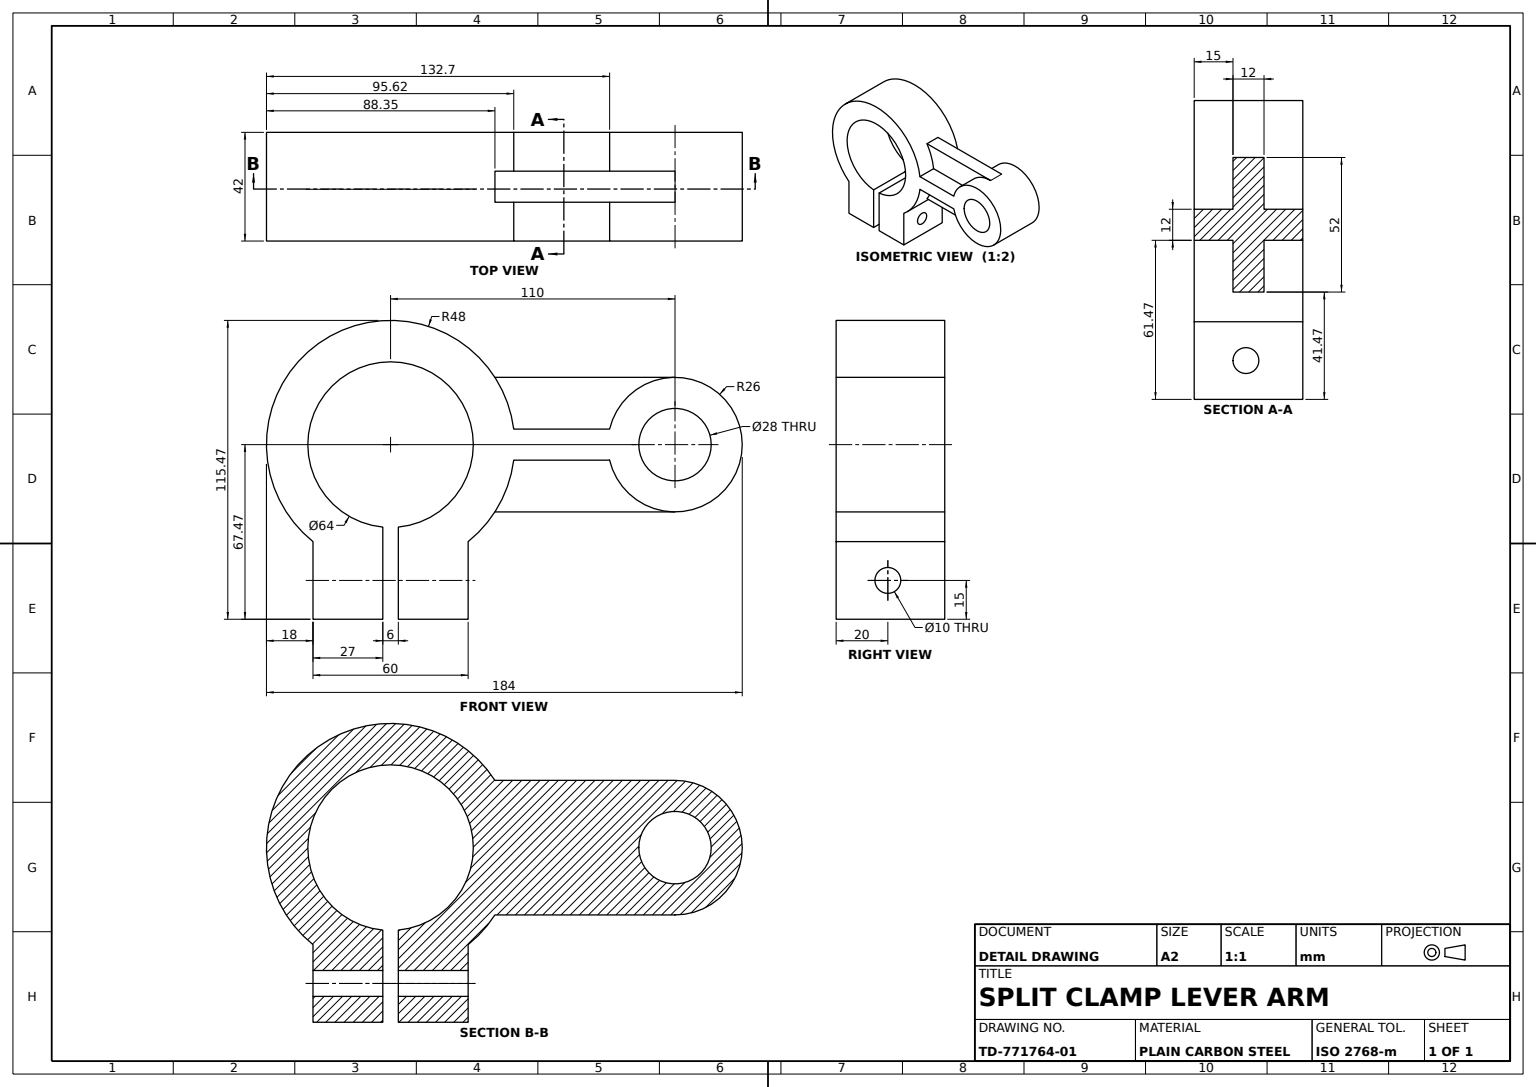
from build123d import *

# Parameters (mm, degrees)
CLAMP_BODY_DEPTH          = 40
CLAMP_BODY_DEPTH_BACK     = 2
CLAMP_SCREW_HOLE_SKETCH_R = 5
CLAMP_SCREW_HOLE_10_DEPTH = 111.617355236
PIVOT_ARM_SKETCH_R        = 14
PIVOT_ARM_AND_BOSS_DEPTH  = 42
ARM_RIB_REACH             = 171.802
ARM_RIB_SKETCH_WALLS_W    = 433.168174749
ARM_RIB_SKETCH_WALLS_H    = 12
CLAMP_RIB_REACH           = 161.912
CLAMP_RIB_SKETCH_WALLS_W  = 402.175841481
CLAMP_RIB_SKETCH_WALLS_H  = 12
BORE_START                = -60
BORE_SKETCH_R             = 32
BORE_64_DEPTH             = 60


with BuildPart() as part:
    # Clamp Body Sketch → Clamp Body (new, two sides: drawn at the far end of the back side and taken through both)
    with BuildSketch(Plane.XY.offset(-CLAMP_BODY_DEPTH_BACK)):
        with BuildLine():
            ThreePointArc((30, -37.46998799), (17.305444592, -44.771883895), (3, -47.906158268))
            Line((3, -47.906158268), (3, -53.969677407))
            Line((3, -53.969677407), (3, -67.46998799))
            Line((3, -67.46998799), (30, -67.46998799))
            Line((30, -67.46998799), (30, -37.46998799))
        make_face()
        with BuildLine():
            ThreePointArc((3, -47.906158268), (0, 48), (-3, -47.906158268))
            Line((-3, -47.906158268), (-3, -31.859064644))
            ThreePointArc((-3, -31.859064644), (0, 32), (3, -31.859064644))
            Line((3, -31.859064644), (3, -47.906158268))
        make_face()
        with BuildLine():
            ThreePointArc((-3, -47.906158268), (-17.305444592, -44.771883895), (-30, -37.46998799))
            Line((-30, -37.46998799), (-30, -67.46998799))
            Line((-30, -67.46998799), (-3, -67.46998799))
            Line((-3, -67.46998799), (-3, -47.906158268))
        make_face()
    extrude(amount=CLAMP_BODY_DEPTH + CLAMP_BODY_DEPTH_BACK)

    # Clamp Screw Hole Sketch → Clamp Screw Hole _10 (cut, through all)
    with BuildSketch(Plane.ZY.offset(30)):
        with Locations((20, -52.46998799)):
            Circle(CLAMP_SCREW_HOLE_SKETCH_R)
    extrude(amount=-CLAMP_SCREW_HOLE_10_DEPTH, mode=Mode.SUBTRACT)

    # Pivot Arm Sketch → Pivot Arm and Boss (add)
    with BuildSketch(Plane.XY.offset(40)):
        with BuildLine():
            Line((40.319786094, 6), (40.319786094, -6))
            Line((40.319786094, -6), (84.701778719, -6))
            ThreePointArc((84.701778719, -6), (136, 0), (84.701778719, 6))
            Line((84.701778719, 6), (40.319786094, 6))
        make_face()
        with Locations((110, 0)):
            Circle(PIVOT_ARM_SKETCH_R, mode=Mode.SUBTRACT)
    extrude(amount=-PIVOT_ARM_AND_BOSS_DEPTH)

    # Arm Rib Sketch walls → Arm Rib (add, up to next)
    with BuildSketch(Plane(origin=(0, 26, 0), x_dir=(1, 0, 0), z_dir=(0, 1, 0)), mode=Mode.PRIVATE) as arm_rib_sk1:
        with Locations((64.5685648, -19)):
            Rectangle(ARM_RIB_SKETCH_WALLS_W, ARM_RIB_SKETCH_WALLS_H)
    arm_rib_tool1 = extrude(arm_rib_sk1.sketch, amount=-ARM_RIB_REACH, mode=Mode.PRIVATE) - part.part
    add(arm_rib_tool1.solids().sort_by_distance((64.568564799, 26, 19))[0])

    # Clamp Rib Sketch walls → Clamp Rib (add, up to next)
    with BuildSketch(Plane(origin=(0, -26, 0), x_dir=(1, 0, 0), z_dir=(0, 1, 0)), mode=Mode.PRIVATE) as clamp_rib_sk1:
        with Locations((70.17544468, -19)):
            Rectangle(CLAMP_RIB_SKETCH_WALLS_W, CLAMP_RIB_SKETCH_WALLS_H)
    clamp_rib_tool1 = extrude(clamp_rib_sk1.sketch, amount=CLAMP_RIB_REACH, mode=Mode.PRIVATE) - part.part
    add(clamp_rib_tool1.solids().sort_by_distance((70.17544468, -26, 19))[0])

    # Bore Sketch → Bore _64 (cut)
    with BuildSketch(Plane.XY.offset(40).offset(BORE_START)):
        Circle(BORE_SKETCH_R)
    extrude(amount=BORE_64_DEPTH, mode=Mode.SUBTRACT)


solid = part.part
